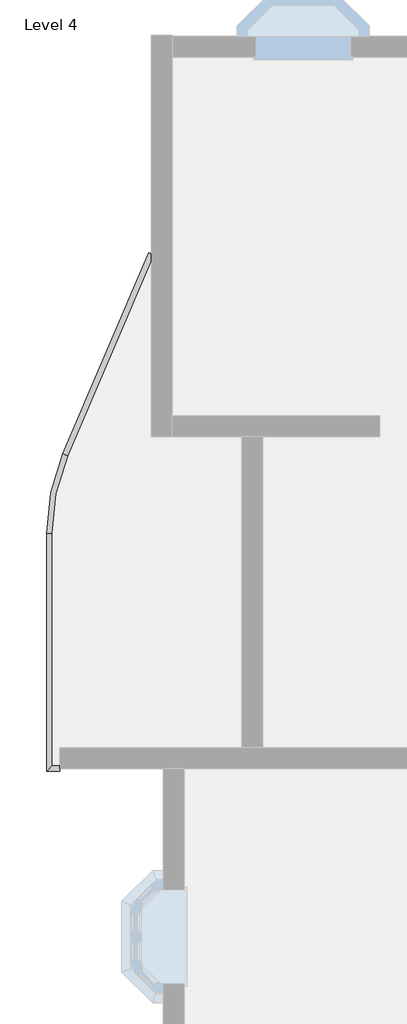
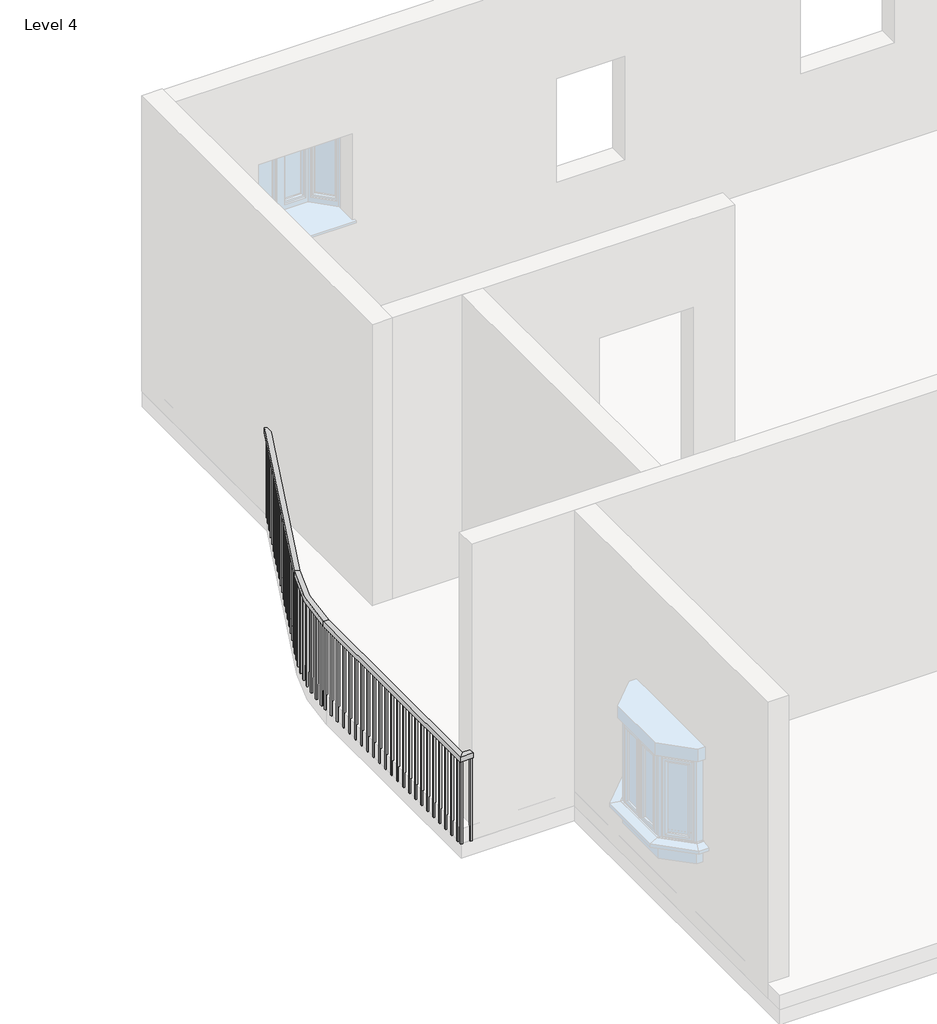
# One storey, part 7 of 14: 1 railing.
"""IFC4 building model written with IfcOpenShell, lengths in millimetres."""

from ifc_helpers import new_model, si_unit, frame, origin, place, context, project, spatial, polyline, circle_curve, outline, extrude, element, save
from ifc_brep_helpers import plane_surface, cylinder_surface, revolved_surface, advanced_brep

model = new_model("IFC4")

# Units and contexts
model_context = context("Model", 3, world=origin())
ifc_project = project(units=[si_unit("LENGTHUNIT", "METRE", prefix="MILLI")], contexts=[model_context])

# Site, building, storey
site = spatial("IfcSite", under=ifc_project)
building = spatial("IfcBuilding", under=site)
storey = spatial("IfcBuildingStorey", under=building, Name="Level 4", Elevation=9144.0)

# Railing
placement = place(None, origin())
element("IfcRailing", 1, ObjectType="Handrail - Rectangular", at=placement, inside=storey, context=model_context, shape_type="SolidModel", body=[
    advanced_brep(
    [(-12381.4379579, -2441.2590879, 10058.4), (-12381.4379579, -2441.2590879, 10007.6), (-12428.1364721, -2421.2618688, 10007.6), (-12428.1364721, -2421.2618688, 10058.4), (-13216.1814979, -4390.5942894, 10058.4), (-13216.1814979, -4390.5942894, 10007.6), (-13262.8800121, -4370.5970703, 10007.6), (-13262.8800121, -4370.5970703, 10058.4), (-13369.987215, -5140.4900045, 10007.6), (-13369.987215, -5140.4900045, 10058.4), (-13420.787215, -5140.4900045, 10007.6), (-13420.787215, -5140.4900045, 10058.4), (-13369.987215, -7396.5416506, 10058.4), (-13369.987215, -7396.5416506, 10007.6), (-13420.787215, -7447.3416506, 10007.6), (-13420.787215, -7447.3416506, 10058.4), (-13293.787215, -7396.5416506, 10058.4), (-13293.787215, -7447.3416506, 10058.4), (-13293.787215, -7447.3416506, 10007.6), (-13293.787215, -7396.5416506, 10007.6)],
    [
        (0, 1),
        (1, 2),
        (2, 3),
        (3, 0),
        (0, 4),
        (4, 5),
        (5, 1),
        (5, 6),
        (6, 2),
        (6, 7),
        (7, 3),
        (7, 4),
        (8, 5, circle_curve(frame((-11464.987215, -5140.4900045, 10007.6), z_axis=(0.0, 0.0, -1.0), x_axis=(-0.9192620907623801, 0.39364604467361003, 0.0)), 1905.0)),
        (4, 9, circle_curve(frame((-11464.987215, -5140.4900045, 10058.4), z_axis=(0.0, 0.0, 1.0), x_axis=(-0.9192620907623801, 0.39364604467361003, 0.0)), 1905.0)),
        (9, 8),
        (10, 6, circle_curve(frame((-11464.987215, -5140.4900045, 10007.6), z_axis=(0.0, 0.0, -1.0), x_axis=(-0.9192620907623801, 0.39364604467361003, 0.0)), 1955.8)),
        (8, 10),
        (11, 7, circle_curve(frame((-11464.987215, -5140.4900045, 10058.4), z_axis=(0.0, 0.0, -1.0), x_axis=(-0.9192620907623801, 0.39364604467361003, 0.0)), 1955.8)),
        (10, 11),
        (11, 9),
        (9, 12),
        (12, 13),
        (13, 8),
        (13, 14),
        (14, 10),
        (14, 15),
        (15, 11),
        (15, 12),
        (16, 17),
        (17, 18),
        (18, 19),
        (19, 16),
        (12, 16),
        (19, 13),
        (18, 14),
        (17, 15),
    ],
    [
        plane_surface(frame((-12404.787215, -2431.2604783, 10058.4), z_axis=(0.39364604467361003, 0.9192620907623801, 0.0), x_axis=(0.9192620907623801, -0.39364604467361003, 0.0))),
        plane_surface(frame((-12381.4379579, -2441.2590879, 10058.4), z_axis=(0.91926209076238, -0.39364604467361014, 0.0), x_axis=(-0.39364604467361014, -0.91926209076238, 0.0))),
        plane_surface(frame((-12381.4379579, -2441.2590879, 10007.6), z_axis=(0.0, 0.0, -1.0), x_axis=(-0.39364604467361014, -0.91926209076238, 0.0))),
        plane_surface(frame((-12428.1364721, -2421.2618688, 10007.6), z_axis=(-0.91926209076238, 0.39364604467361014, 0.0), x_axis=(-0.39364604467361014, -0.91926209076238, 0.0))),
        plane_surface(frame((-12428.1364721, -2421.2618688, 10058.4), z_axis=(0.0, 0.0, 1.0), x_axis=(-0.39364604467361014, -0.91926209076238, 0.0))),
        revolved_surface(polyline([(-13216.181497902333, -4390.594289396773, 10058.4), (-13216.181497902333, -4390.594289396773, 10007.6)]), (-11464.987215, -5140.4900045, 10058.4), (0.0, 0.0, 1.0)),
        plane_surface(frame((-11464.987215, -5140.4900045, 10007.6), z_axis=(0.0, 0.0, -1.0000000000000002), x_axis=(-0.9192620907623801, 0.39364604467361003, 0.0))),
        cylinder_surface(frame((-11464.987215, -5140.4900045, 10058.4), z_axis=(0.0, 0.0, 1.0), x_axis=(-0.9192620907623801, 0.39364604467361003, 0.0)), 1955.8),
        plane_surface(frame((-11464.987215, -5140.4900045, 10058.4), z_axis=(0.0, 0.0, 1.0000000000000002), x_axis=(-0.9192620907623801, 0.39364604467361003, 0.0))),
        plane_surface(frame((-13369.987215, -5140.4900045, 10058.4), z_axis=(1.0, 0.0, 0.0), x_axis=(0.0, -1.0, 0.0))),
        plane_surface(frame((-13369.987215, -5140.4900045, 10007.6), z_axis=(0.0, 0.0, -1.0), x_axis=(0.0, -1.0, 0.0))),
        plane_surface(frame((-13420.787215, -5140.4900045, 10007.6), z_axis=(-1.0, 0.0, 0.0), x_axis=(0.0, -1.0, 0.0))),
        plane_surface(frame((-13420.787215, -5140.4900045, 10058.4), z_axis=(0.0, 0.0, 1.0), x_axis=(0.0, -1.0, 0.0))),
        plane_surface(frame((-13293.787215, -7421.9416506, 10058.4), z_axis=(1.0, 0.0, 0.0), x_axis=(0.0, 1.0, 0.0))),
        plane_surface(frame((-13369.987215, -7396.5416506, 10058.4), z_axis=(0.0, 1.0, 0.0), x_axis=(1.0, 0.0, 0.0))),
        plane_surface(frame((-13369.987215, -7396.5416506, 10007.6), z_axis=(0.0, 0.0, -1.0), x_axis=(1.0, 0.0, 0.0))),
        plane_surface(frame((-13420.787215, -7447.3416506, 10007.6), z_axis=(0.0, -1.0, 0.0), x_axis=(1.0, 0.0, 0.0))),
        plane_surface(frame((-13420.787215, -7447.3416506, 10058.4), z_axis=(0.0, 0.0, 1.0), x_axis=(1.0, 0.0, 0.0))),
    ],
    [
        (0, [[1, 2, 3, 4]]),
        (1, [[-1, 5, 6, 7]]),
        (2, [[-2, -7, 8, 9]]),
        (3, [[-3, -9, 10, 11]]),
        (4, [[-4, -11, 12, -5]]),
        (5, [[13, -6, 14, 15]]),
        (6, [[16, -8, -13, 17]]),
        (7, [[18, -10, -16, 19]]),
        (8, [[-14, -12, -18, 20]]),
        (9, [[-15, 21, 22, 23]]),
        (10, [[-17, -23, 24, 25]]),
        (11, [[-19, -25, 26, 27]]),
        (12, [[-20, -27, 28, -21]]),
        (13, [[29, 30, 31, 32]]),
        (14, [[-22, 33, -32, 34]]),
        (15, [[-24, -34, -31, 35]]),
        (16, [[-26, -35, -30, 36]]),
        (17, [[-28, -36, -29, -33]]),
    ],
),
    extrude(outline(polyline([(-13404.912215, -7366.1650045), (-13385.862215, -7366.1650045), (-13385.862215, -7385.2150045), (-13404.912215, -7385.2150045), (-13404.912215, -7366.1650045)])), frame((0.0, 0.0, 9144.0), z_axis=(0.0, 0.0, 1.0), x_axis=(1.0, 0.0, 0.0)), (0.0, 0.0, 1.0), 863.6),
    extrude(outline(polyline([(-13404.912215, -7264.5650045), (-13385.862215, -7264.5650045), (-13385.862215, -7283.6150045), (-13404.912215, -7283.6150045), (-13404.912215, -7264.5650045)])), frame((0.0, 0.0, 9144.0), z_axis=(0.0, 0.0, 1.0), x_axis=(1.0, 0.0, 0.0)), (0.0, 0.0, 1.0), 863.6),
    extrude(outline(polyline([(-13404.912215, -7162.9650045), (-13385.862215, -7162.9650045), (-13385.862215, -7182.0150045), (-13404.912215, -7182.0150045), (-13404.912215, -7162.9650045)])), frame((0.0, 0.0, 9144.0), z_axis=(0.0, 0.0, 1.0), x_axis=(1.0, 0.0, 0.0)), (0.0, 0.0, 1.0), 863.6),
    extrude(outline(polyline([(-13404.912215, -7061.3650045), (-13385.862215, -7061.3650045), (-13385.862215, -7080.4150045), (-13404.912215, -7080.4150045), (-13404.912215, -7061.3650045)])), frame((0.0, 0.0, 9144.0), z_axis=(0.0, 0.0, 1.0), x_axis=(1.0, 0.0, 0.0)), (0.0, 0.0, 1.0), 863.6),
    extrude(outline(polyline([(-13404.912215, -6959.7650045), (-13385.862215, -6959.7650045), (-13385.862215, -6978.8150045), (-13404.912215, -6978.8150045), (-13404.912215, -6959.7650045)])), frame((0.0, 0.0, 9144.0), z_axis=(0.0, 0.0, 1.0), x_axis=(1.0, 0.0, 0.0)), (0.0, 0.0, 1.0), 863.6),
    extrude(outline(polyline([(-13404.912215, -6858.1650045), (-13385.862215, -6858.1650045), (-13385.862215, -6877.2150045), (-13404.912215, -6877.2150045), (-13404.912215, -6858.1650045)])), frame((0.0, 0.0, 9144.0), z_axis=(0.0, 0.0, 1.0), x_axis=(1.0, 0.0, 0.0)), (0.0, 0.0, 1.0), 863.6),
    extrude(outline(polyline([(-13404.912215, -6756.5650045), (-13385.862215, -6756.5650045), (-13385.862215, -6775.6150045), (-13404.912215, -6775.6150045), (-13404.912215, -6756.5650045)])), frame((0.0, 0.0, 9144.0), z_axis=(0.0, 0.0, 1.0), x_axis=(1.0, 0.0, 0.0)), (0.0, 0.0, 1.0), 863.6),
    extrude(outline(polyline([(-13404.912215, -6654.9650045), (-13385.862215, -6654.9650045), (-13385.862215, -6674.0150045), (-13404.912215, -6674.0150045), (-13404.912215, -6654.9650045)])), frame((0.0, 0.0, 9144.0), z_axis=(0.0, 0.0, 1.0), x_axis=(1.0, 0.0, 0.0)), (0.0, 0.0, 1.0), 863.6),
    extrude(outline(polyline([(-13404.912215, -6553.3650045), (-13385.862215, -6553.3650045), (-13385.862215, -6572.4150045), (-13404.912215, -6572.4150045), (-13404.912215, -6553.3650045)])), frame((0.0, 0.0, 9144.0), z_axis=(0.0, 0.0, 1.0), x_axis=(1.0, 0.0, 0.0)), (0.0, 0.0, 1.0), 863.6),
    extrude(outline(polyline([(-13404.912215, -6451.7650045), (-13385.862215, -6451.7650045), (-13385.862215, -6470.8150045), (-13404.912215, -6470.8150045), (-13404.912215, -6451.7650045)])), frame((0.0, 0.0, 9144.0), z_axis=(0.0, 0.0, 1.0), x_axis=(1.0, 0.0, 0.0)), (0.0, 0.0, 1.0), 863.6),
    extrude(outline(polyline([(-13404.912215, -6350.1650045), (-13385.862215, -6350.1650045), (-13385.862215, -6369.2150045), (-13404.912215, -6369.2150045), (-13404.912215, -6350.1650045)])), frame((0.0, 0.0, 9144.0), z_axis=(0.0, 0.0, 1.0), x_axis=(1.0, 0.0, 0.0)), (0.0, 0.0, 1.0), 863.6),
    extrude(outline(polyline([(-13404.912215, -6248.5650045), (-13385.862215, -6248.5650045), (-13385.862215, -6267.6150045), (-13404.912215, -6267.6150045), (-13404.912215, -6248.5650045)])), frame((0.0, 0.0, 9144.0), z_axis=(0.0, 0.0, 1.0), x_axis=(1.0, 0.0, 0.0)), (0.0, 0.0, 1.0), 863.6),
    extrude(outline(polyline([(-13404.912215, -6146.9650045), (-13385.862215, -6146.9650045), (-13385.862215, -6166.0150045), (-13404.912215, -6166.0150045), (-13404.912215, -6146.9650045)])), frame((0.0, 0.0, 9144.0), z_axis=(0.0, 0.0, 1.0), x_axis=(1.0, 0.0, 0.0)), (0.0, 0.0, 1.0), 863.6),
    extrude(outline(polyline([(-13404.912215, -6045.3650045), (-13385.862215, -6045.3650045), (-13385.862215, -6064.4150045), (-13404.912215, -6064.4150045), (-13404.912215, -6045.3650045)])), frame((0.0, 0.0, 9144.0), z_axis=(0.0, 0.0, 1.0), x_axis=(1.0, 0.0, 0.0)), (0.0, 0.0, 1.0), 863.6),
    extrude(outline(polyline([(-13404.912215, -5943.7650045), (-13385.862215, -5943.7650045), (-13385.862215, -5962.8150045), (-13404.912215, -5962.8150045), (-13404.912215, -5943.7650045)])), frame((0.0, 0.0, 9144.0), z_axis=(0.0, 0.0, 1.0), x_axis=(1.0, 0.0, 0.0)), (0.0, 0.0, 1.0), 863.6),
    extrude(outline(polyline([(-13404.912215, -5842.1650045), (-13385.862215, -5842.1650045), (-13385.862215, -5861.2150045), (-13404.912215, -5861.2150045), (-13404.912215, -5842.1650045)])), frame((0.0, 0.0, 9144.0), z_axis=(0.0, 0.0, 1.0), x_axis=(1.0, 0.0, 0.0)), (0.0, 0.0, 1.0), 863.6),
    extrude(outline(polyline([(-13404.912215, -5740.5650045), (-13385.862215, -5740.5650045), (-13385.862215, -5759.6150045), (-13404.912215, -5759.6150045), (-13404.912215, -5740.5650045)])), frame((0.0, 0.0, 9144.0), z_axis=(0.0, 0.0, 1.0), x_axis=(1.0, 0.0, 0.0)), (0.0, 0.0, 1.0), 863.6),
    extrude(outline(polyline([(-13404.912215, -5638.9650045), (-13385.862215, -5638.9650045), (-13385.862215, -5658.0150045), (-13404.912215, -5658.0150045), (-13404.912215, -5638.9650045)])), frame((0.0, 0.0, 9144.0), z_axis=(0.0, 0.0, 1.0), x_axis=(1.0, 0.0, 0.0)), (0.0, 0.0, 1.0), 863.6),
    extrude(outline(polyline([(-13404.912215, -5537.3650045), (-13385.862215, -5537.3650045), (-13385.862215, -5556.4150045), (-13404.912215, -5556.4150045), (-13404.912215, -5537.3650045)])), frame((0.0, 0.0, 9144.0), z_axis=(0.0, 0.0, 1.0), x_axis=(1.0, 0.0, 0.0)), (0.0, 0.0, 1.0), 863.6),
    extrude(outline(polyline([(-13404.912215, -5435.7650045), (-13385.862215, -5435.7650045), (-13385.862215, -5454.8150045), (-13404.912215, -5454.8150045), (-13404.912215, -5435.7650045)])), frame((0.0, 0.0, 9144.0), z_axis=(0.0, 0.0, 1.0), x_axis=(1.0, 0.0, 0.0)), (0.0, 0.0, 1.0), 863.6),
    extrude(outline(polyline([(-13404.912215, -5334.1650045), (-13385.862215, -5334.1650045), (-13385.862215, -5353.2150045), (-13404.912215, -5353.2150045), (-13404.912215, -5334.1650045)])), frame((0.0, 0.0, 9144.0), z_axis=(0.0, 0.0, 1.0), x_axis=(1.0, 0.0, 0.0)), (0.0, 0.0, 1.0), 863.6),
    extrude(outline(polyline([(-13404.912215, -5232.5650045), (-13385.862215, -5232.5650045), (-13385.862215, -5251.6150045), (-13404.912215, -5251.6150045), (-13404.912215, -5232.5650045)])), frame((0.0, 0.0, 9144.0), z_axis=(0.0, 0.0, 1.0), x_axis=(1.0, 0.0, 0.0)), (0.0, 0.0, 1.0), 863.6),
    extrude(outline(polyline([(-13403.2986616, -5060.8127369), (-13384.2611239, -5061.5016911), (-13384.9500781, -5080.5392288), (-13403.9876158, -5079.8502746), (-13403.2986616, -5060.8127369)])), frame((0.0, 0.0, 9144.0), z_axis=(0.0, 0.0, 1.0), x_axis=(1.0, 0.0, 0.0)), (0.0, 0.0, 1.0), 863.6),
    extrude(outline(polyline([(-13396.4230348, -4958.9537683), (-13377.4481028, -4960.6432816), (-13379.1376161, -4979.6182136), (-13398.1125481, -4977.9287003), (-13396.4230348, -4958.9537683)])), frame((0.0, 0.0, 9144.0), z_axis=(0.0, 0.0, 1.0), x_axis=(1.0, 0.0, 0.0)), (0.0, 0.0, 1.0), 863.6),
    extrude(outline(polyline([(-13384.1984052, -4857.5975541), (-13365.3386289, -4860.2829475), (-13368.0240223, -4879.1427238), (-13386.8837986, -4876.4573304), (-13384.1984052, -4857.5975541)])), frame((0.0, 0.0, 9144.0), z_axis=(0.0, 0.0, 1.0), x_axis=(1.0, 0.0, 0.0)), (0.0, 0.0, 1.0), 863.6),
    extrude(outline(polyline([(-13366.6586282, -4757.0247946), (-13347.9662387, -4760.698631), (-13351.6400752, -4779.3910205), (-13370.3324647, -4775.7171841), (-13366.6586282, -4757.0247946)])), frame((0.0, 0.0, 9144.0), z_axis=(0.0, 0.0, 1.0), x_axis=(1.0, 0.0, 0.0)), (0.0, 0.0, 1.0), 863.6),
    extrude(outline(polyline([(-13343.8522793, -4657.5140204), (-13325.3790441, -4662.1661254), (-13330.0311492, -4680.6393606), (-13348.5043844, -4675.9872556), (-13343.8522793, -4657.5140204)])), frame((0.0, 0.0, 9144.0), z_axis=(0.0, 0.0, 1.0), x_axis=(1.0, 0.0, 0.0)), (0.0, 0.0, 1.0), 863.6),
    extrude(outline(polyline([(-13315.8425193, -4559.340821), (-13297.6395991, -4564.9583109), (-13303.257089, -4583.1612312), (-13321.4600093, -4577.5437413), (-13315.8425193, -4559.340821)])), frame((0.0, 0.0, 9144.0), z_axis=(0.0, 0.0, 1.0), x_axis=(1.0, 0.0, 0.0)), (0.0, 0.0, 1.0), 863.6),
    extrude(outline(polyline([(-13282.7069198, -4462.7770815), (-13264.8247264, -4469.344399), (-13271.3920438, -4487.2265924), (-13289.2742372, -4480.659275), (-13282.7069198, -4462.7770815)])), frame((0.0, 0.0, 9144.0), z_axis=(0.0, 0.0, 1.0), x_axis=(1.0, 0.0, 0.0)), (0.0, 0.0, 1.0), 863.6),
    extrude(outline(polyline([(-13209.6824706, -4286.6955968), (-13192.1705278, -4294.1945539), (-13199.6694849, -4311.7064967), (-13217.1814277, -4304.2075396), (-13209.6824706, -4286.6955968)])), frame((0.0, 0.0, 9144.0), z_axis=(0.0, 0.0, 1.0), x_axis=(1.0, 0.0, 0.0)), (0.0, 0.0, 1.0), 863.6),
    extrude(outline(polyline([(-13169.6880325, -4193.2985683), (-13152.1760896, -4200.7975255), (-13159.6750468, -4218.3094683), (-13177.1869896, -4210.8105112), (-13169.6880325, -4193.2985683)])), frame((0.0, 0.0, 9144.0), z_axis=(0.0, 0.0, 1.0), x_axis=(1.0, 0.0, 0.0)), (0.0, 0.0, 1.0), 863.6),
    extrude(outline(polyline([(-13129.6935943, -4099.9015399), (-13112.1816515, -4107.4004971), (-13119.6806086, -4124.9124399), (-13137.1925515, -4117.4134827), (-13129.6935943, -4099.9015399)])), frame((0.0, 0.0, 9144.0), z_axis=(0.0, 0.0, 1.0), x_axis=(1.0, 0.0, 0.0)), (0.0, 0.0, 1.0), 863.6),
    extrude(outline(polyline([(-13089.6991562, -4006.5045115), (-13072.1872133, -4014.0034686), (-13079.6861705, -4031.5154115), (-13097.1981133, -4024.0164543), (-13089.6991562, -4006.5045115)])), frame((0.0, 0.0, 9144.0), z_axis=(0.0, 0.0, 1.0), x_axis=(1.0, 0.0, 0.0)), (0.0, 0.0, 1.0), 863.6),
    extrude(outline(polyline([(-13049.704718, -3913.1074831), (-13032.1927752, -3920.6064402), (-13039.6917324, -3938.1183831), (-13057.2036752, -3930.6194259), (-13049.704718, -3913.1074831)])), frame((0.0, 0.0, 9144.0), z_axis=(0.0, 0.0, 1.0), x_axis=(1.0, 0.0, 0.0)), (0.0, 0.0, 1.0), 863.6),
    extrude(outline(polyline([(-13009.7102799, -3819.7104546), (-12992.1983371, -3827.2094118), (-12999.6972942, -3844.7213546), (-13017.209237, -3837.2223975), (-13009.7102799, -3819.7104546)])), frame((0.0, 0.0, 9144.0), z_axis=(0.0, 0.0, 1.0), x_axis=(1.0, 0.0, 0.0)), (0.0, 0.0, 1.0), 863.6),
    extrude(outline(polyline([(-12969.7158418, -3726.3134262), (-12952.2038989, -3733.8123834), (-12959.7028561, -3751.3243262), (-12977.2147989, -3743.8253691), (-12969.7158418, -3726.3134262)])), frame((0.0, 0.0, 9144.0), z_axis=(0.0, 0.0, 1.0), x_axis=(1.0, 0.0, 0.0)), (0.0, 0.0, 1.0), 863.6),
    extrude(outline(polyline([(-12929.7214036, -3632.9163978), (-12912.2094608, -3640.415355), (-12919.7084179, -3657.9272978), (-12937.2203608, -3650.4283406), (-12929.7214036, -3632.9163978)])), frame((0.0, 0.0, 9144.0), z_axis=(0.0, 0.0, 1.0), x_axis=(1.0, 0.0, 0.0)), (0.0, 0.0, 1.0), 863.6),
    extrude(outline(polyline([(-12889.7269655, -3539.5193694), (-12872.2150227, -3547.0183265), (-12879.7139798, -3564.5302694), (-12897.2259226, -3557.0313122), (-12889.7269655, -3539.5193694)])), frame((0.0, 0.0, 9144.0), z_axis=(0.0, 0.0, 1.0), x_axis=(1.0, 0.0, 0.0)), (0.0, 0.0, 1.0), 863.6),
    extrude(outline(polyline([(-12849.7325273, -3446.122341), (-12832.2205845, -3453.6212981), (-12839.7195417, -3471.1332409), (-12857.2314845, -3463.6342838), (-12849.7325273, -3446.122341)])), frame((0.0, 0.0, 9144.0), z_axis=(0.0, 0.0, 1.0), x_axis=(1.0, 0.0, 0.0)), (0.0, 0.0, 1.0), 863.6),
    extrude(outline(polyline([(-12809.7380892, -3352.7253125), (-12792.2261464, -3360.2242697), (-12799.7251035, -3377.7362125), (-12817.2370464, -3370.2372554), (-12809.7380892, -3352.7253125)])), frame((0.0, 0.0, 9144.0), z_axis=(0.0, 0.0, 1.0), x_axis=(1.0, 0.0, 0.0)), (0.0, 0.0, 1.0), 863.6),
    extrude(outline(polyline([(-12769.7436511, -3259.3282841), (-12752.2317082, -3266.8272413), (-12759.7306654, -3284.3391841), (-12777.2426082, -3276.8402269), (-12769.7436511, -3259.3282841)])), frame((0.0, 0.0, 9144.0), z_axis=(0.0, 0.0, 1.0), x_axis=(1.0, 0.0, 0.0)), (0.0, 0.0, 1.0), 863.6),
    extrude(outline(polyline([(-12729.7492129, -3165.9312557), (-12712.2372701, -3173.4302129), (-12719.7362272, -3190.9421557), (-12737.2481701, -3183.4431985), (-12729.7492129, -3165.9312557)])), frame((0.0, 0.0, 9144.0), z_axis=(0.0, 0.0, 1.0), x_axis=(1.0, 0.0, 0.0)), (0.0, 0.0, 1.0), 863.6),
    extrude(outline(polyline([(-12689.7547748, -3072.5342273), (-12672.242832, -3080.0331844), (-12679.7417891, -3097.5451273), (-12697.2537319, -3090.0461701), (-12689.7547748, -3072.5342273)])), frame((0.0, 0.0, 9144.0), z_axis=(0.0, 0.0, 1.0), x_axis=(1.0, 0.0, 0.0)), (0.0, 0.0, 1.0), 863.6),
    extrude(outline(polyline([(-12649.7603366, -2979.1371989), (-12632.2483938, -2986.636156), (-12639.747351, -3004.1480988), (-12657.2592938, -2996.6491417), (-12649.7603366, -2979.1371989)])), frame((0.0, 0.0, 9144.0), z_axis=(0.0, 0.0, 1.0), x_axis=(1.0, 0.0, 0.0)), (0.0, 0.0, 1.0), 863.6),
    extrude(outline(polyline([(-12609.7658985, -2885.7401704), (-12592.2539557, -2893.2391276), (-12599.7529128, -2910.7510704), (-12617.2648557, -2903.2521133), (-12609.7658985, -2885.7401704)])), frame((0.0, 0.0, 9144.0), z_axis=(0.0, 0.0, 1.0), x_axis=(1.0, 0.0, 0.0)), (0.0, 0.0, 1.0), 863.6),
    extrude(outline(polyline([(-12569.7714604, -2792.343142), (-12552.2595175, -2799.8420992), (-12559.7584747, -2817.354042), (-12577.2704175, -2809.8550848), (-12569.7714604, -2792.343142)])), frame((0.0, 0.0, 9144.0), z_axis=(0.0, 0.0, 1.0), x_axis=(1.0, 0.0, 0.0)), (0.0, 0.0, 1.0), 863.6),
    extrude(outline(polyline([(-12529.7770222, -2698.9461136), (-12512.2650794, -2706.4450707), (-12519.7640366, -2723.9570136), (-12537.2759794, -2716.4580564), (-12529.7770222, -2698.9461136)])), frame((0.0, 0.0, 9144.0), z_axis=(0.0, 0.0, 1.0), x_axis=(1.0, 0.0, 0.0)), (0.0, 0.0, 1.0), 863.6),
    extrude(outline(polyline([(-12489.7825841, -2605.5490852), (-12472.2706413, -2613.0480423), (-12479.7695984, -2630.5599852), (-12497.2815412, -2623.061028), (-12489.7825841, -2605.5490852)])), frame((0.0, 0.0, 9144.0), z_axis=(0.0, 0.0, 1.0), x_axis=(1.0, 0.0, 0.0)), (0.0, 0.0, 1.0), 863.6),
    extrude(outline(polyline([(-12449.788146, -2512.1520567), (-12432.2762031, -2519.6510139), (-12439.7751603, -2537.1629567), (-12457.2871031, -2529.6639996), (-12449.788146, -2512.1520567)])), frame((0.0, 0.0, 9144.0), z_axis=(0.0, 0.0, 1.0), x_axis=(1.0, 0.0, 0.0)), (0.0, 0.0, 1.0), 863.6),
    extrude(outline(polyline([(-13404.912215, -7412.4166506), (-13385.862215, -7412.4166506), (-13385.862215, -7431.4666506), (-13404.912215, -7431.4666506), (-13404.912215, -7412.4166506)])), frame((0.0, 0.0, 9144.0), z_axis=(0.0, 0.0, 1.0), x_axis=(1.0, 0.0, 0.0)), (0.0, 0.0, 1.0), 863.6),
    extrude(outline(polyline([(-13404.912215, -5130.9650045), (-13385.862215, -5130.9650045), (-13385.862215, -5150.0150045), (-13404.912215, -5150.0150045), (-13404.912215, -5130.9650045)])), frame((0.0, 0.0, 9144.0), z_axis=(0.0, 0.0, 1.0), x_axis=(1.0, 0.0, 0.0)), (0.0, 0.0, 1.0), 863.6),
    extrude(outline(polyline([(-13244.5372478, -4368.0902299), (-13227.025305, -4375.589187), (-13234.5242621, -4393.1011299), (-13252.036205, -4385.6021727), (-13244.5372478, -4368.0902299)])), frame((0.0, 0.0, 9144.0), z_axis=(0.0, 0.0, 1.0), x_axis=(1.0, 0.0, 0.0)), (0.0, 0.0, 1.0), 863.6),
    extrude(outline(polyline([(-13312.837215, -7431.4666506), (-13312.837215, -7412.4166506), (-13293.787215, -7412.4166506), (-13293.787215, -7431.4666506), (-13312.837215, -7431.4666506)])), frame((0.0, 0.0, 9144.0), z_axis=(0.0, 0.0, 1.0), x_axis=(1.0, 0.0, 0.0)), (0.0, 0.0, 1.0), 863.6),
    extrude(outline(polyline([(-12413.5431864, -2427.5109997), (-12396.0312436, -2435.0099569), (-12403.5302007, -2452.5218997), (-12421.0421435, -2445.0229426), (-12413.5431864, -2427.5109997)])), frame((0.0, 0.0, 9144.0), z_axis=(0.0, 0.0, 1.0), x_axis=(1.0, 0.0, 0.0)), (0.0, 0.0, 1.0), 863.6),
])

save(model, "model.ifc")

# Revit data of these elements
# Type "Handrail - Rectangular"
#   Assembly Code = "C2010400"
#   built-in parameter 1008612 = 0.0416667 (stored number, unit not read)
#   built-in parameter 1008611 = 0.0416667 (stored number, unit not read)
#   built-in parameter 1008609 = 0.333333 (stored number, unit not read)
#   built-in parameter 1008604 = 0.166667 (stored number, unit not read)
#   built-in parameter 1008603 = 0.166667 (stored number, unit not read)
#   Railing Height = 3' - 0"
#   built-in parameter 1008630 = 2
#   built-in parameter 1008610 = 2
#   built-in parameter 1008618 = Baluster - Square : 3/4"
# Element 1 (IfcRailing, "Handrail - Rectangular")
#   Phase Created = New Construction
